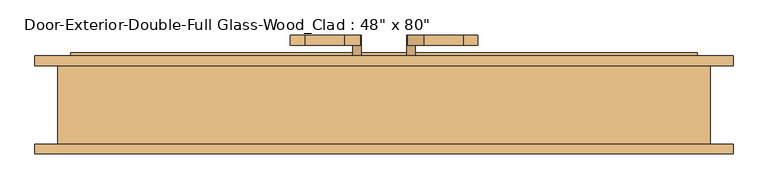
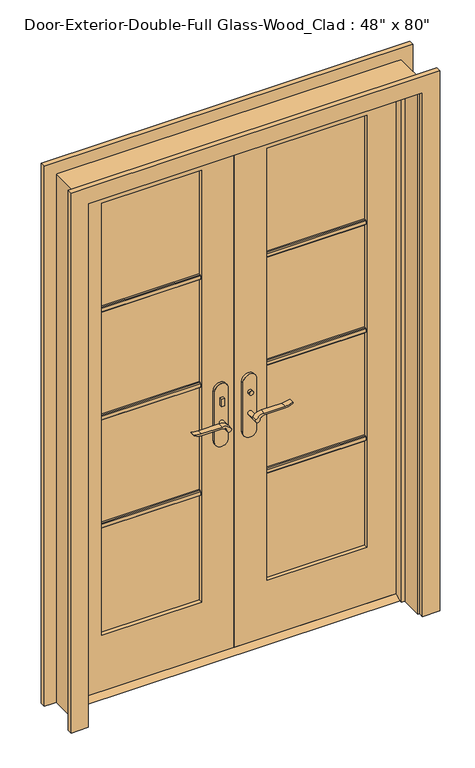
"""IFC4 building model written with IfcOpenShell, lengths in millimetres: door geometry."""

from ifc_helpers import new_model, si_unit, point, frame, frame_2d, origin, place, context, project, spatial, polyline, circle_curve, trimmed, segment, composite_curve, outline, extrude, faceted_brep, source, transform, mapped, element, save


def door_3efe7946(model_context):
    return source(origin(), model_context, "Body", "SolidModel", [
        extrude(outline(polyline([(38.1, 12.7), (73.025, 12.7), (98.425, 0.0), (12.7, 0.0), (38.1, 12.7)])), frame((-609.6, 0.0, 0.0), z_axis=(1.0, 0.0, 0.0), x_axis=(0.0, 1.0, 0.0)), (0.0, 0.0, 1.0), 1219.2),
        extrude(outline(polyline([(-47.4019111, 18.1), (-57.4019111, 18.1), (-57.4019111, 28.1), (-47.4019111, 28.1), (-47.4019111, 18.1)])), frame((0.0, 0.0, 981.9), z_axis=(0.0, 0.0, 1.0), x_axis=(1.0, 0.0, 0.0)), (0.0, 0.0, 1.0), 30.0),
        extrude(outline(composite_curve([segment(trimmed(circle_curve(frame_2d((996.9, -52.4019111)), 8.0), [point((996.9, -60.4019111))], [point((996.9, -44.4019111))], False, "CARTESIAN"), True, "CONTINUOUS"), segment(trimmed(circle_curve(frame_2d((996.9, -52.4019111)), 8.0), [point((996.9, -44.4019111))], [point((996.9, -60.4019111))], False, "CARTESIAN"), True, "CONTINUOUS")], self_intersect=False)), frame((0.0, 83.025, 0.0), z_axis=(0.0, 1.0, 0.0), x_axis=(0.0, 0.0, 1.0)), (0.0, 0.0, 1.0), 10.0),
        extrude(outline(composite_curve([segment(trimmed(circle_curve(frame_2d((897.1555521, -76.0694241)), 37.2832219), [point((919.0523287, -45.8937749))], [point((934.4, -77.7693445))], False, "CARTESIAN"), True, "CONTINUOUS"), segment(polyline([(934.4, -77.7693445), (934.4, -154.045502)]), True, "CONTINUOUS"), segment(trimmed(circle_curve(frame_2d((1017.6850638, -153.9791202)), 83.2850902), [point((934.4, -154.045502))], [point((939.4, -182.4019111))], True, "CARTESIAN"), True, "CONTINUOUS"), segment(polyline([(939.4, -182.4019111), (936.6135558, -182.4019111)]), True, "CONTINUOUS"), segment(trimmed(circle_curve(frame_2d((986.6709207, -150.4622499)), 59.3791355), [point((936.6135558, -182.4019111))], [point((927.4, -154.045502))], False, "CARTESIAN"), True, "CONTINUOUS"), segment(polyline([(927.4, -154.045502), (927.4, -77.7881013)]), True, "CONTINUOUS"), segment(trimmed(circle_curve(frame_2d((909.2738613, -77.7881013)), 18.1261387), [point((927.4, -77.7881013))], [point((914.4, -60.4019111))], True, "CARTESIAN"), True, "CONTINUOUS"), segment(trimmed(circle_curve(frame_2d((914.4, -52.4019111)), 8.0), [point((914.4, -60.4019111))], [point((919.0523287, -45.8937749))], False, "CARTESIAN"), True, "CONTINUOUS")], self_intersect=False)), frame((0.0, -21.9, 0.0), z_axis=(0.0, 1.0, 0.0), x_axis=(0.0, 0.0, 1.0)), (0.0, 0.0, 1.0), 20.0),
        extrude(outline(composite_curve([segment(trimmed(circle_curve(frame_2d((914.4, -52.4019111)), 8.0), [point((914.3999903, -60.4019111))], [point((919.0523287, -45.8937749))], False, "CARTESIAN"), True, "CONTINUOUS"), segment(trimmed(circle_curve(frame_2d((897.1555521, -76.0694241)), 37.2832219), [point((919.0523287, -45.8937749))], [point((934.4, -77.7693445))], False, "CARTESIAN"), True, "CONTINUOUS"), segment(polyline([(934.4, -77.7693445), (934.4, -154.045502)]), True, "CONTINUOUS"), segment(trimmed(circle_curve(frame_2d((1017.6850638, -153.9791202)), 83.2850902), [point((934.4, -154.045502))], [point((939.4, -182.4019111))], True, "CARTESIAN"), True, "CONTINUOUS"), segment(polyline([(939.4, -182.4019111), (936.6135558, -182.4019111)]), True, "CONTINUOUS"), segment(trimmed(circle_curve(frame_2d((986.6709207, -150.4622499)), 59.3791355), [point((936.6135558, -182.4019111))], [point((927.4, -154.045502))], False, "CARTESIAN"), True, "CONTINUOUS"), segment(polyline([(927.4, -154.045502), (927.4, -77.788099)]), True, "CONTINUOUS"), segment(trimmed(circle_curve(frame_2d((909.2738682, -77.788099)), 18.1261318), [point((927.4, -77.788099))], [point((914.3999903, -60.4019111))], True, "CARTESIAN"), True, "CONTINUOUS")], self_intersect=False)), frame((0.0, 113.025, 0.0), z_axis=(0.0, 1.0, 0.0), x_axis=(0.0, 0.0, 1.0)), (0.0, 0.0, 1.0), 20.0),
        extrude(outline(composite_curve([segment(trimmed(circle_curve(frame_2d((914.4, -52.4019111)), 8.0), [point((914.4, -60.4019111))], [point((914.4, -44.4019111))], False, "CARTESIAN"), True, "CONTINUOUS"), segment(trimmed(circle_curve(frame_2d((914.4, -52.4019111)), 8.0), [point((914.4, -44.4019111))], [point((914.4, -60.4019111))], False, "CARTESIAN"), True, "CONTINUOUS")], self_intersect=False)), frame((0.0, -1.9, 0.0), z_axis=(0.0, 1.0, 0.0), x_axis=(0.0, 0.0, 1.0)), (0.0, 0.0, 1.0), 30.0),
        extrude(outline(composite_curve([segment(trimmed(circle_curve(frame_2d((914.4, -52.4019111)), 8.0), [point((914.4, -60.4019111))], [point((914.4, -44.4019111))], False, "CARTESIAN"), True, "CONTINUOUS"), segment(trimmed(circle_curve(frame_2d((914.4, -52.4019111)), 8.0), [point((914.4, -44.4019111))], [point((914.4, -60.4019111))], False, "CARTESIAN"), True, "CONTINUOUS")], self_intersect=False)), frame((0.0, 83.025, 0.0), z_axis=(0.0, 1.0, 0.0), x_axis=(0.0, 0.0, 1.0)), (0.0, 0.0, 1.0), 30.0),
        extrude(outline(composite_curve([segment(polyline([(844.4, -27.4019111), (1039.4, -27.4019111)]), True, "CONTINUOUS"), segment(trimmed(circle_curve(frame_2d((1039.4, -52.4019111)), 25.0), [point((1039.4, -27.4019111))], [point((1039.4, -77.4019111))], False, "CARTESIAN"), True, "CONTINUOUS"), segment(polyline([(1039.4, -77.4019111), (844.4, -77.4019111)]), True, "CONTINUOUS"), segment(trimmed(circle_curve(frame_2d((844.4, -52.4019111)), 25.0), [point((844.4, -77.4019111))], [point((844.4, -27.4019111))], False, "CARTESIAN"), True, "CONTINUOUS")], self_intersect=False)), frame((0.0, 28.1, 0.0), z_axis=(0.0, 1.0, 0.0), x_axis=(0.0, 0.0, 1.0)), (0.0, 0.0, 1.0), 10.0),
        extrude(outline(composite_curve([segment(polyline([(844.4, -27.4019111), (1039.4, -27.4019111)]), True, "CONTINUOUS"), segment(trimmed(circle_curve(frame_2d((1039.4, -52.4019111)), 25.0), [point((1039.4, -27.4019111))], [point((1039.4, -77.4019111))], False, "CARTESIAN"), True, "CONTINUOUS"), segment(polyline([(1039.4, -77.4019111), (844.4, -77.4019111)]), True, "CONTINUOUS"), segment(trimmed(circle_curve(frame_2d((844.4, -52.4019111)), 25.0), [point((844.4, -77.4019111))], [point((844.4, -27.4019111))], False, "CARTESIAN"), True, "CONTINUOUS")], self_intersect=False)), frame((0.0, 73.025, 0.0), z_axis=(0.0, 1.0, 0.0), x_axis=(0.0, 0.0, 1.0)), (0.0, 0.0, 1.0), 10.0),
        extrude(outline(polyline([(47.3875, 93.025), (57.3875, 93.025), (57.3875, 83.025), (47.3875, 83.025), (47.3875, 93.025)])), frame((0.0, 0.0, 981.9), z_axis=(0.0, 0.0, 1.0), x_axis=(1.0, 0.0, 0.0)), (0.0, 0.0, 1.0), 30.0),
        extrude(outline(composite_curve([segment(trimmed(circle_curve(frame_2d((996.9, 52.3875)), 8.0), [point((996.9, 60.3875))], [point((996.9, 44.3875))], False, "CARTESIAN"), True, "CONTINUOUS"), segment(trimmed(circle_curve(frame_2d((996.9, 52.3875)), 8.0), [point((996.9, 44.3875))], [point((996.9, 60.3875))], False, "CARTESIAN"), True, "CONTINUOUS")], self_intersect=False)), frame((0.0, 18.1, 0.0), z_axis=(0.0, 1.0, 0.0), x_axis=(0.0, 0.0, 1.0)), (0.0, 0.0, 1.0), 10.0),
        extrude(outline(composite_curve([segment(trimmed(circle_curve(frame_2d((914.4, 52.3875)), 8.0), [point((919.0523287, 45.8793637))], [point((914.4, 60.3875))], False, "CARTESIAN"), True, "CONTINUOUS"), segment(trimmed(circle_curve(frame_2d((909.2738613, 77.7736901)), 18.1261387), [point((914.4, 60.3875))], [point((927.4, 77.7736901))], True, "CARTESIAN"), True, "CONTINUOUS"), segment(polyline([(927.4, 77.7736901), (927.4, 154.0310909)]), True, "CONTINUOUS"), segment(trimmed(circle_curve(frame_2d((986.6709207, 150.4478388)), 59.3791355), [point((927.4, 154.0310909))], [point((936.6135558, 182.3875))], False, "CARTESIAN"), True, "CONTINUOUS"), segment(polyline([(936.6135558, 182.3875), (939.4, 182.3875)]), True, "CONTINUOUS"), segment(trimmed(circle_curve(frame_2d((1017.6850638, 153.9647091)), 83.2850902), [point((939.4, 182.3875))], [point((934.4, 154.0310909))], True, "CARTESIAN"), True, "CONTINUOUS"), segment(polyline([(934.4, 154.0310909), (934.4, 77.7549333)]), True, "CONTINUOUS"), segment(trimmed(circle_curve(frame_2d((897.1555521, 76.0550129)), 37.2832219), [point((934.4, 77.7549333))], [point((919.0523287, 45.8793637))], False, "CARTESIAN"), True, "CONTINUOUS")], self_intersect=False)), frame((0.0, 113.025, 0.0), z_axis=(0.0, 1.0, 0.0), x_axis=(0.0, 0.0, 1.0)), (0.0, 0.0, 1.0), 20.0),
        extrude(outline(composite_curve([segment(trimmed(circle_curve(frame_2d((909.2738682, 77.7736878)), 18.1261318), [point((914.3999903, 60.3875))], [point((927.4, 77.7736878))], True, "CARTESIAN"), True, "CONTINUOUS"), segment(polyline([(927.4, 77.7736878), (927.4, 154.0310909)]), True, "CONTINUOUS"), segment(trimmed(circle_curve(frame_2d((986.6709207, 150.4478388)), 59.3791355), [point((927.4, 154.0310909))], [point((936.6135558, 182.3875))], False, "CARTESIAN"), True, "CONTINUOUS"), segment(polyline([(936.6135558, 182.3875), (939.4, 182.3875)]), True, "CONTINUOUS"), segment(trimmed(circle_curve(frame_2d((1017.6850638, 153.9647091)), 83.2850902), [point((939.4, 182.3875))], [point((934.4, 154.0310909))], True, "CARTESIAN"), True, "CONTINUOUS"), segment(polyline([(934.4, 154.0310909), (934.4, 77.7549333)]), True, "CONTINUOUS"), segment(trimmed(circle_curve(frame_2d((897.1555521, 76.0550129)), 37.2832219), [point((934.4, 77.7549333))], [point((919.0523287, 45.8793637))], False, "CARTESIAN"), True, "CONTINUOUS"), segment(trimmed(circle_curve(frame_2d((914.4, 52.3875)), 8.0), [point((919.0523287, 45.8793637))], [point((914.3999903, 60.3875))], False, "CARTESIAN"), True, "CONTINUOUS")], self_intersect=False)), frame((0.0, -21.9, 0.0), z_axis=(0.0, 1.0, 0.0), x_axis=(0.0, 0.0, 1.0)), (0.0, 0.0, 1.0), 20.0),
        extrude(outline(composite_curve([segment(trimmed(circle_curve(frame_2d((914.4, 52.3875)), 8.0), [point((914.4, 60.3875))], [point((914.4, 44.3875))], False, "CARTESIAN"), True, "CONTINUOUS"), segment(trimmed(circle_curve(frame_2d((914.4, 52.3875)), 8.0), [point((914.4, 44.3875))], [point((914.4, 60.3875))], False, "CARTESIAN"), True, "CONTINUOUS")], self_intersect=False)), frame((0.0, 83.025, 0.0), z_axis=(0.0, 1.0, 0.0), x_axis=(0.0, 0.0, 1.0)), (0.0, 0.0, 1.0), 30.0),
        extrude(outline(composite_curve([segment(trimmed(circle_curve(frame_2d((914.4, 52.3875)), 8.0), [point((914.4, 60.3875))], [point((914.4, 44.3875))], False, "CARTESIAN"), True, "CONTINUOUS"), segment(trimmed(circle_curve(frame_2d((914.4, 52.3875)), 8.0), [point((914.4, 44.3875))], [point((914.4, 60.3875))], False, "CARTESIAN"), True, "CONTINUOUS")], self_intersect=False)), frame((0.0, -1.9, 0.0), z_axis=(0.0, 1.0, 0.0), x_axis=(0.0, 0.0, 1.0)), (0.0, 0.0, 1.0), 30.0),
        extrude(outline(composite_curve([segment(trimmed(circle_curve(frame_2d((844.4, 52.3875)), 25.0), [point((844.4, 27.3875))], [point((844.4, 77.3875))], False, "CARTESIAN"), True, "CONTINUOUS"), segment(polyline([(844.4, 77.3875), (1039.4, 77.3875)]), True, "CONTINUOUS"), segment(trimmed(circle_curve(frame_2d((1039.4, 52.3875)), 25.0), [point((1039.4, 77.3875))], [point((1039.4, 27.3875))], False, "CARTESIAN"), True, "CONTINUOUS"), segment(polyline([(1039.4, 27.3875), (844.4, 27.3875)]), True, "CONTINUOUS")], self_intersect=False)), frame((0.0, 73.025, 0.0), z_axis=(0.0, 1.0, 0.0), x_axis=(0.0, 0.0, 1.0)), (0.0, 0.0, 1.0), 10.0),
        extrude(outline(composite_curve([segment(trimmed(circle_curve(frame_2d((844.4, 52.3875)), 25.0), [point((844.4, 27.3875))], [point((844.4, 77.3875))], False, "CARTESIAN"), True, "CONTINUOUS"), segment(polyline([(844.4, 77.3875), (1039.4, 77.3875)]), True, "CONTINUOUS"), segment(trimmed(circle_curve(frame_2d((1039.4, 52.3875)), 25.0), [point((1039.4, 77.3875))], [point((1039.4, 27.3875))], False, "CARTESIAN"), True, "CONTINUOUS"), segment(polyline([(1039.4, 27.3875), (844.4, 27.3875)]), True, "CONTINUOUS")], self_intersect=False)), frame((0.0, 28.1, 0.0), z_axis=(0.0, 1.0, 0.0), x_axis=(0.0, 0.0, 1.0)), (0.0, 0.0, 1.0), 10.0),
        extrude(outline(polyline([(52.07, 1502.171875), (52.07, 1483.121875), (45.72, 1483.121875), (42.545, 1486.296875), (42.545, 1498.996875), (45.72, 1502.171875), (52.07, 1502.171875)])), frame((120.65, 0.0, 0.0), z_axis=(1.0, 0.0, 0.0), x_axis=(0.0, 1.0, 0.0)), (0.0, 0.0, 1.0), 368.3),
        extrude(outline(polyline([(52.07, 1081.88125), (52.07, 1062.83125), (45.72, 1062.83125), (42.545, 1066.00625), (42.545, 1078.70625), (45.72, 1081.88125), (52.07, 1081.88125)])), frame((120.65, 0.0, 0.0), z_axis=(1.0, 0.0, 0.0), x_axis=(0.0, 1.0, 0.0)), (0.0, 0.0, 1.0), 368.3),
        extrude(outline(polyline([(52.07, 661.590625), (52.07, 642.540625), (45.72, 642.540625), (42.545, 645.715625), (42.545, 658.415625), (45.72, 661.590625), (52.07, 661.590625)])), frame((120.65, 0.0, 0.0), z_axis=(1.0, 0.0, 0.0), x_axis=(0.0, 1.0, 0.0)), (0.0, 0.0, 1.0), 368.3),
        extrude(outline(polyline([(59.055, 1502.171875), (65.405, 1502.171875), (68.58, 1498.996875), (68.58, 1486.296875), (65.405, 1483.121875), (59.055, 1483.121875), (59.055, 1502.171875)])), frame((-488.95, 0.0, 0.0), z_axis=(1.0, 0.0, 0.0), x_axis=(0.0, 1.0, 0.0)), (0.0, 0.0, 1.0), 368.3),
        extrude(outline(polyline([(59.055, 1081.88125), (65.405, 1081.88125), (68.58, 1078.70625), (68.58, 1066.00625), (65.405, 1062.83125), (59.055, 1062.83125), (59.055, 1081.88125)])), frame((-488.95, 0.0, 0.0), z_axis=(1.0, 0.0, 0.0), x_axis=(0.0, 1.0, 0.0)), (0.0, 0.0, 1.0), 368.3),
        extrude(outline(polyline([(59.055, 661.590625), (65.405, 661.590625), (68.58, 658.415625), (68.58, 645.715625), (65.405, 642.540625), (59.055, 642.540625), (59.055, 661.590625)])), frame((-488.95, 0.0, 0.0), z_axis=(1.0, 0.0, 0.0), x_axis=(0.0, 1.0, 0.0)), (0.0, 0.0, 1.0), 368.3),
        extrude(outline(polyline([(59.055, 1502.171875), (65.405, 1502.171875), (68.58, 1498.996875), (68.58, 1486.296875), (65.405, 1483.121875), (59.055, 1483.121875), (59.055, 1502.171875)])), frame((120.65, 0.0, 0.0), z_axis=(1.0, 0.0, 0.0), x_axis=(0.0, 1.0, 0.0)), (0.0, 0.0, 1.0), 368.3),
        extrude(outline(polyline([(59.055, 1081.88125), (65.405, 1081.88125), (68.58, 1078.70625), (68.58, 1066.00625), (65.405, 1062.83125), (59.055, 1062.83125), (59.055, 1081.88125)])), frame((120.65, 0.0, 0.0), z_axis=(1.0, 0.0, 0.0), x_axis=(0.0, 1.0, 0.0)), (0.0, 0.0, 1.0), 368.3),
        extrude(outline(polyline([(59.055, 661.590625), (65.405, 661.590625), (68.58, 658.415625), (68.58, 645.715625), (65.405, 642.540625), (59.055, 642.540625), (59.055, 661.590625)])), frame((120.65, 0.0, 0.0), z_axis=(1.0, 0.0, 0.0), x_axis=(0.0, 1.0, 0.0)), (0.0, 0.0, 1.0), 368.3),
        extrude(outline(polyline([(52.07, 1502.171875), (52.07, 1483.121875), (45.72, 1483.121875), (42.545, 1486.296875), (42.545, 1498.996875), (45.72, 1502.171875), (52.07, 1502.171875)])), frame((-488.95, 0.0, 0.0), z_axis=(1.0, 0.0, 0.0), x_axis=(0.0, 1.0, 0.0)), (0.0, 0.0, 1.0), 368.3),
        extrude(outline(polyline([(52.07, 1081.88125), (52.07, 1062.83125), (45.72, 1062.83125), (42.545, 1066.00625), (42.545, 1078.70625), (45.72, 1081.88125), (52.07, 1081.88125)])), frame((-488.95, 0.0, 0.0), z_axis=(1.0, 0.0, 0.0), x_axis=(0.0, 1.0, 0.0)), (0.0, 0.0, 1.0), 368.3),
        extrude(outline(polyline([(52.07, 661.590625), (52.07, 642.540625), (45.72, 642.540625), (42.545, 645.715625), (42.545, 658.415625), (45.72, 661.590625), (52.07, 661.590625)])), frame((-488.95, 0.0, 0.0), z_axis=(1.0, 0.0, 0.0), x_axis=(0.0, 1.0, 0.0)), (0.0, 0.0, 1.0), 368.3),
        extrude(outline(polyline([(0.0, 615.95), (0.0, 679.45), (2101.85, 679.45), (2101.85, -679.45), (0.0, -679.45), (0.0, -615.95), (2038.35, -615.95), (2038.35, 615.95), (0.0, 615.95)])), frame((0.0, 73.025, 0.0), z_axis=(0.0, 1.0, 0.0), x_axis=(0.0, 0.0, 1.0)), (0.0, 0.0, 1.0), 19.05),
        extrude(outline(polyline([(0.0, 615.95), (0.0, 679.45), (2101.85, 679.45), (2101.85, -679.45), (0.0, -679.45), (0.0, -615.95), (2038.35, -615.95), (2038.35, 615.95), (0.0, 615.95)])), frame((0.0, -98.425, 0.0), z_axis=(0.0, 1.0, 0.0), x_axis=(0.0, 0.0, 1.0)), (0.0, 0.0, 1.0), 19.05),
        extrude(outline(polyline([(12.7, 609.6), (2032.0, 609.6), (2032.0, 1.5875), (12.7, 1.5875), (12.7, 609.6)]), holes=[polyline([(1912.9375, 120.65), (1912.9375, 488.95), (231.775, 488.95), (231.775, 120.65), (1912.9375, 120.65)])]), frame((0.0, 38.1, 0.0), z_axis=(0.0, 1.0, 0.0), x_axis=(0.0, 0.0, 1.0)), (0.0, 0.0, 1.0), 34.925),
        extrude(outline(polyline([(2032.0, -609.6), (12.7, -609.6), (12.7, -1.6019111), (2032.0, -1.6019111), (2032.0, -609.6)]), holes=[polyline([(231.775, -488.95), (1912.9375, -488.95), (1912.9375, -120.65), (231.775, -120.65), (231.775, -488.95)])]), frame((0.0, 38.1, 0.0), z_axis=(0.0, 1.0, 0.0), x_axis=(0.0, 0.0, 1.0)), (0.0, 0.0, 1.0), 34.925),
        faceted_brep([(635.0, 73.025, 0.0), (635.0, -79.375, 0.0), (609.6, -79.375, 0.0), (609.6, 3.175, 0.0), (596.9, 3.175, 0.0), (596.9, 38.1, 0.0), (609.6, 38.1, 0.0), (609.6, 73.025, 0.0), (635.0, 73.025, 2057.4), (635.0, -79.375, 2057.4), (-635.0, -79.375, 2057.4), (-635.0, -79.375, 0.0), (-609.6, -79.375, 0.0), (-609.6, -79.375, 2032.0), (609.6, -79.375, 2032.0), (609.6, 3.175, 2032.0), (-609.6, 3.175, 2032.0), (-609.6, 3.175, 0.0), (-596.9, 3.175, 0.0), (-596.9, 3.175, 2019.3), (596.9, 3.175, 2019.3), (596.9, 38.1, 2019.3), (1.5875, 38.1, 2019.3), (-1.6019111, 38.1, 2019.3), (-596.9, 38.1, 2019.3), (-596.9, 38.1, 0.0), (-609.6, 38.1, 0.0), (-609.6, 38.1, 2032.0), (-1.6019111, 38.1, 2032.0), (1.5875, 38.1, 2032.0), (609.6, 38.1, 2032.0), (609.6, 73.025, 2032.0), (1.5875, 73.025, 2032.0), (-1.6019111, 73.025, 2032.0), (-609.6, 73.025, 2032.0), (-609.6, 73.025, 0.0), (-635.0, 73.025, 0.0), (-635.0, 73.025, 2057.4)], [[[0, 1, 2, 3, 4, 5, 6, 7]], [[1, 0, 8, 9]], [[2, 1, 9, 10, 11, 12, 13, 14]], [[3, 2, 14, 15]], [[4, 3, 15, 16, 17, 18, 19, 20]], [[5, 4, 20, 21]], [[6, 5, 21, 22, 23, 24, 25, 26, 27, 28, 29, 30]], [[7, 6, 30, 31]], [[0, 7, 31, 32, 33, 34, 35, 36, 37, 8]], [[9, 8, 37, 10]], [[14, 13, 16, 15]], [[20, 19, 24, 23, 22, 21]], [[31, 30, 29, 28, 27, 34, 33, 32]], [[12, 11, 36, 35, 26, 25, 18, 17]], [[11, 10, 37, 36]], [[13, 12, 17, 16]], [[19, 18, 25, 24]], [[27, 26, 35, 34]]]),
        extrude(outline(polyline([(488.95, 52.07), (120.65, 52.07), (120.65, 59.055), (488.95, 59.055), (488.95, 52.07)])), frame((0.0, 0.0, 231.775), z_axis=(0.0, 0.0, 1.0), x_axis=(1.0, 0.0, 0.0)), (0.0, 0.0, 1.0), 1681.1625),
        extrude(outline(polyline([(-120.65, 52.07), (-488.95, 52.07), (-488.95, 59.055), (-120.65, 59.055), (-120.65, 52.07)])), frame((0.0, 0.0, 231.775), z_axis=(0.0, 0.0, 1.0), x_axis=(1.0, 0.0, 0.0)), (0.0, 0.0, 1.0), 1681.1625),
    ])


if __name__ == "__main__":
    model = new_model("IFC4")
    model_context = context("Model", 3, world=origin())
    ifc_project = project(units=[si_unit("LENGTHUNIT", "METRE", prefix="MILLI")], contexts=[model_context])
    site = spatial("IfcSite", under=ifc_project)
    building = spatial("IfcBuilding", under=site)
    placement = place(None, origin())
    door_shape = door_3efe7946(model_context)
    element("IfcDoor", 1, ObjectType="Door-Exterior-Double-Full Glass-Wood_Clad : 48\" x 80\"", at=placement, inside=building, context=model_context, shape_type="MappedRepresentation", body=[
        mapped(door_shape, transform((0.0, 0.0, 0.0), x_axis=(1.0, 0.0, 0.0), y_axis=(0.0, 1.0, 0.0), z_axis=(0.0, 0.0, 1.0))),
    ])
    save(model, "model.ifc")

# Revit data of these elements
# Type "Door-Exterior-Double-Full Glass-Wood_Clad : 48\" x 80\""
#   Type Mark = "8"
#   Assembly Code = "B2030100"
#   Analytic Construction = "French door, wood frame with double glass"
#   Top Rail = 0' - 4 11/16"
#   Threshold Offset [instance default] = 0' - 0 1/2"
#   Thickness = 0' - 1 3/8"
#   Thermal Resistance (R) = 1.9158 (h·ft²·°F)/BTU
#   Swing Angle [instance default] = 90.00°
#   Stiles = 0' - 4 3/4"
#   Rough Width = 4' - 2"
#   Rough Height = 6' - 9"
#   Panel Width = 2' - 0"
#   Door Offset [instance default] = 0' - 0"
#   Height = 6' - 8"
#   Width = 4' - 0"
#   Heat Transfer Coefficient (U) = 0.5220 BTU/(h·ft²·°F)
#   Bottom Rail = 0' - 9 1/8"
#   Exterior Trim [instance default] = yes
#   Threshold [instance default] = yes
#   Show Grill [instance default] = yes
#   Function = 1
#   Trim Material = Cherry
#   Threshold Material = Cherry
#   Panel Material = Cherry
#   Glazing = Glass
#   Frame Material = Cherry
#   Door Handle Material = Aluminum
#   Visual Light Transmittance = 0
#   Solar Heat Gain Coefficient = 0
#   Wall Closure = (empty or 0)
#   Construction Type = (empty or 0)
# Element 1 (IfcDoor, "Door-Exterior-Double-Full Glass-Wood_Clad : 48\" x 80\"")
#   Materials on its faces: "Cherry", "Aluminum", "Glass"
# Materials
#   "Cherry": class "Wood", colour RGB 226 177 128, transparency 0, Description = "Prunus Serotina", Cost = 0
#   "Glass": class "Glass", colour RGB 0 128 192, transparency 0.75, Description = "Soda Lime Glass", Cost = 0
#   "Aluminum": class "Metal", colour RGB 247 247 247, transparency 0, Description = "Aluminum 6061", Cost = 0
